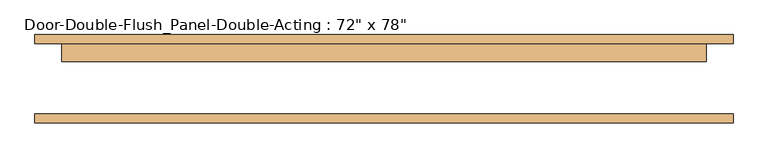
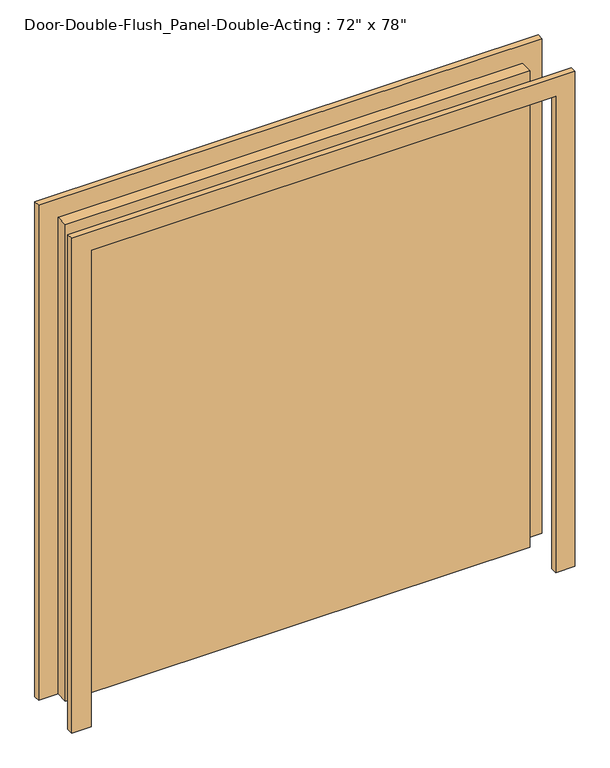
"""IFC4 building model written with IfcOpenShell, lengths in millimetres: door geometry."""

from ifc_helpers import new_model, si_unit, frame, origin, origin_with_axes, place, context, project, spatial, polyline, outline, extrude, source, transform, mapped, element, save


def door_8409b21c(model_context):
    return source(origin(), model_context, "Body", "SweptSolid", [
        extrude(outline(polyline([(2057.4, -990.6), (0.0, -990.6), (0.0, -914.4), (1981.2, -914.4), (1981.2, 914.4), (0.0, 914.4), (0.0, 990.6), (2057.4, 990.6), (2057.4, -990.6)])), frame((0.0, 100.0, 0.0), z_axis=(0.0, 1.0, 0.0), x_axis=(0.0, 0.0, 1.0)), (0.0, 0.0, 1.0), 25.4),
        extrude(outline(polyline([(1981.2, -914.4), (1981.2, 914.4), (0.0, 914.4), (0.0, 990.6), (2057.4, 990.6), (2057.4, -990.6), (0.0, -990.6), (0.0, -914.4), (1981.2, -914.4)])), frame((0.0, -125.4, 0.0), z_axis=(0.0, 1.0, 0.0), x_axis=(0.0, 0.0, 1.0)), (0.0, 0.0, 1.0), 25.4),
        extrude(outline(polyline([(-914.4, 100.0), (914.4, 100.0), (914.4, 49.2), (-914.4, 49.2), (-914.4, 100.0)])), origin_with_axes(), (0.0, 0.0, 1.0), 1981.2),
    ])


if __name__ == "__main__":
    model = new_model("IFC4")
    model_context = context("Model", 3, world=origin())
    ifc_project = project(units=[si_unit("LENGTHUNIT", "METRE", prefix="MILLI")], contexts=[model_context])
    site = spatial("IfcSite", under=ifc_project)
    building = spatial("IfcBuilding", under=site)
    placement = place(None, origin())
    door_shape = door_8409b21c(model_context)
    element("IfcDoor", 1, ObjectType="Door-Double-Flush_Panel-Double-Acting : 72\" x 78\"", at=placement, inside=building, context=model_context, shape_type="MappedRepresentation", body=[
        mapped(door_shape, transform((0.0, 0.0, 0.0), x_axis=(1.0, 0.0, 0.0), y_axis=(0.0, 1.0, 0.0), z_axis=(0.0, 0.0, 1.0))),
    ])
    save(model, "model.ifc")

# Revit data of these elements
# Type "Door-Double-Flush_Panel-Double-Acting : 72\" x 78\""
#   Type Mark = "22"
#   Construction Type Id = "DOOR"
#   Assembly Code = "C1020"
#   Analytic Construction = "Wooden"
#   W = 3' - 0"
#   Thickness = 0' - 2"
#   Thermal Resistance (R) = 0.455703 (m²·K)/W
#   Swing Angle [instance default] = 90.00°
#   Heat Transfer Coefficient (U) = 2.19465 W/(m²·K)
#   Height = 6' - 6"
#   Trim Projection Ext. = 0' - 1"
#   Trim Projection Int. = 0' - 1"
#   Trim Width Ext. = 0' - 3"
#   Trim Width Int. = 0' - 3"
#   Width = 6' - 0"
#   Define Thermal Properties by = 1
#   Panel Material = Wood - Birch - Solid Stained Light Low Gloss
#   Trim Material = Paint - Sienna
#   Visual Light Transmittance = 0
#   Solar Heat Gain Coefficient = 0
#   Function = (empty or 0)
#   Wall Closure = (empty or 0)
# Element 1 (IfcDoor, "Door-Double-Flush_Panel-Double-Acting : 72\" x 78\"")
#   Materials on its faces: "Paint - Sienna", "Wood - Birch - Solid Stained Light Low Gloss"
# Materials
#   "Wood - Birch - Solid Stained Light Low Gloss": class "Wood", colour RGB 210 159 95, transparency 0, Cost = 0
#   "Paint - Sienna": colour RGB 118 70 51, transparency 0, Cost = 0
